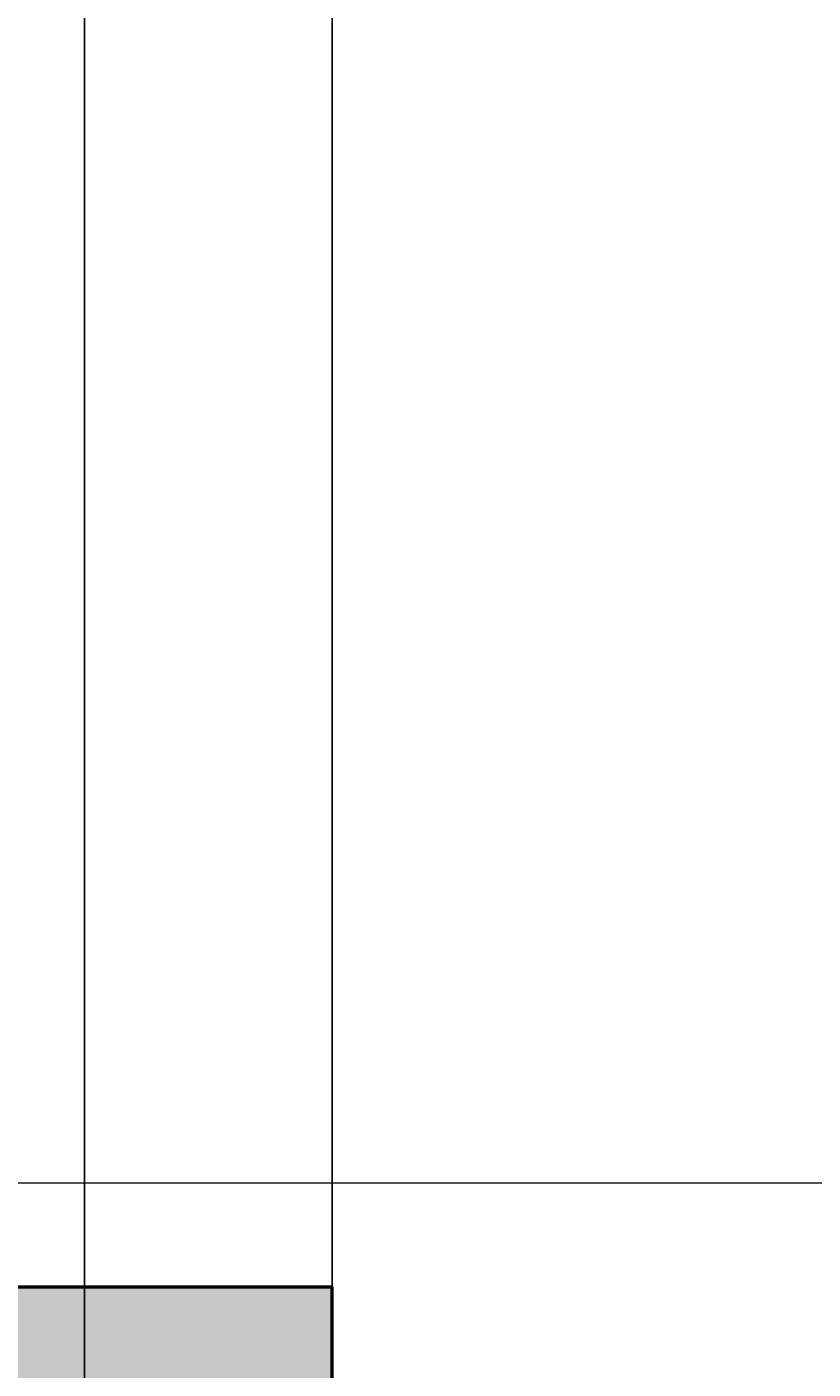
# Model space of a CAD drawing. Units: inches. Extents: x 2231 to 2461, y 2045 to 2455.
# Tile 43 of 95: x 2297 to 2316, y 2185 to 2217. Entities that reach past the tile are written whole.
import ezdxf

# ---------------------------------------------------------------- set-up
doc = ezdxf.new("R2010")
doc.units = ezdxf.units.IN
for name, color, linetype, lineweight in [('A-ANNO-DIMS', 2, 'Continuous', 18), ('A-DOOR', 3, 'Continuous', 25), ('A-FURN', 9, 'Continuous', 18), ('A-WALL', 7, 'Continuous', 50)]:
    doc.layers.add(name, color=color, linetype=linetype, lineweight=lineweight)
doc.layers.add('A-WALL-PATT', color=18, linetype='Continuous', lineweight=13, true_color=0x000000)
doc.styles.get("Standard").update_dxf_attribs({"font": 'arial.ttf'})
doc.dimstyles.get("Standard").update_dxf_attribs({"dimtxt": 0.18, "dimasz": 0.18, "dimexe": 0.18, "dimexo": 0.0625, "dimgap": 0.09, "dimtad": 0, "dimtih": 1, "dimtoh": 1, "dimdec": 4, "dimzin": 0, "dimdsep": 46, "dimtxsty": 'Standard', "dimcen": 0.09, "dimadec": 0, "dimazin": 0, "dimtfac": 1, "dimtdec": 4, "dimtofl": 0, "dimtmove": 0, "dimatfit": 3, "dimfxl": 1, "dimtolj": 1, "dimtzin": 0, "dimarcsym": 0})

# ---------------------------------------------------------------- blocks, each defined once
blk = doc.blocks.new('*U4')
for p, q in [((0, 0), (0, 6)), ((40, 0), (40, 6))]:
    blk.add_line(p, q)
blk.add_lwpolyline([(0, 0), (34.641, -20), (35.516, -18.484), (0.875, 1.516)], close=True)
blk.add_arc((0, 0), 40, 330, 0)
blk = doc.blocks.new('*D49')
at = {"layer": 'A-ANNO-DIMS', "color": 0, "lineweight": -2, "transparency": 16777216}
for p, q in [((2298.794, 2182.895), (2298.794, 2454.645)), ((2304.794, 2182.895), (2304.794, 2454.645)), ((2298.974, 2454.465), (2301.644, 2454.465)), ((2304.614, 2454.465), (2301.943, 2454.465))]:
    blk.add_line(p, q, dxfattribs=at)
at = {"layer": 'A-ANNO-DIMS', "color": 0, "transparency": 16777216}
for points in [[(2298.974, 2454.495), (2298.974, 2454.435), (2298.794, 2454.465)], [(2304.614, 2454.495), (2304.614, 2454.435), (2304.794, 2454.465)]]:
    blk.add_solid(points, dxfattribs=at)
at = {"layer": 'Defpoints', "color": 0, "transparency": 16777216}
for p in [(2304.794, 2454.465), (2298.794, 2182.833), (2304.794, 2182.833)]:
    blk.add_point(p, dxfattribs=at)
at = {"layer": 'A-ANNO-DIMS', "color": 0, "transparency": 16777216, "insert": (2301.794, 2454.465), "char_height": 0.18, "attachment_point": 5}
blk.add_mtext('\\A1;6', dxfattribs=at)
blk = doc.blocks.new('*D50')
at = {"layer": 'A-ANNO-DIMS', "color": 0, "lineweight": -2, "transparency": 16777216}
for p, q in [((2304.794, 2182.895), (2304.794, 2454.645)), ((2334.794, 2182.895), (2334.794, 2454.645)), ((2304.974, 2454.465), (2319.575, 2454.465)), ((2334.614, 2454.465), (2320.012, 2454.465))]:
    blk.add_line(p, q, dxfattribs=at)
at = {"layer": 'A-ANNO-DIMS', "color": 0, "transparency": 16777216}
for points in [[(2304.974, 2454.495), (2304.974, 2454.435), (2304.794, 2454.465)], [(2334.614, 2454.495), (2334.614, 2454.435), (2334.794, 2454.465)]]:
    blk.add_solid(points, dxfattribs=at)
at = {"layer": 'Defpoints', "color": 0, "transparency": 16777216}
for p in [(2334.794, 2454.465), (2304.794, 2182.833), (2334.794, 2182.833)]:
    blk.add_point(p, dxfattribs=at)
at = {"layer": 'A-ANNO-DIMS', "color": 0, "transparency": 16777216, "insert": (2319.794, 2454.465), "char_height": 0.18, "attachment_point": 5}
blk.add_mtext('\\A1;30', dxfattribs=at)
blk = doc.blocks.new('*D51')
at = {"layer": 'A-ANNO-DIMS', "color": 0, "lineweight": -2, "transparency": 16777216}
for p, q in [((2258.794, 2306.77), (2258.794, 2044.803)), ((2330.794, 2306.77), (2330.794, 2044.803)), ((2258.974, 2044.983), (2294.576, 2044.983)), ((2330.614, 2044.983), (2295.011, 2044.983))]:
    blk.add_line(p, q, dxfattribs=at)
at = {"layer": 'A-ANNO-DIMS', "color": 0, "transparency": 16777216}
for points in [[(2258.974, 2045.013), (2258.974, 2044.953), (2258.794, 2044.983)], [(2330.614, 2045.013), (2330.614, 2044.953), (2330.794, 2044.983)]]:
    blk.add_solid(points, dxfattribs=at)
at = {"layer": 'Defpoints', "color": 0, "transparency": 16777216}
for p in [(2258.794, 2306.833), (2330.794, 2306.833), (2330.794, 2044.983)]:
    blk.add_point(p, dxfattribs=at)
at = {"layer": 'A-ANNO-DIMS', "color": 0, "transparency": 16777216, "insert": (2294.794, 2044.983), "char_height": 0.18, "attachment_point": 5}
blk.add_mtext('\\A1;72', dxfattribs=at)
blk = doc.blocks.new('*D65')
at = {"layer": 'A-ANNO-DIMS', "color": 0, "lineweight": -2, "transparency": 16777216}
for p, q in [((2285.635, 2189.285), (2285.635, 2044.803)), ((2340.667, 2189.285), (2340.667, 2044.803)), ((2285.815, 2044.983), (2312.758, 2044.983)), ((2340.487, 2044.983), (2313.545, 2044.983))]:
    blk.add_line(p, q, dxfattribs=at)
at = {"layer": 'A-ANNO-DIMS', "color": 0, "transparency": 16777216}
for points in [[(2285.815, 2045.013), (2285.815, 2044.953), (2285.635, 2044.983)], [(2340.487, 2045.013), (2340.487, 2044.953), (2340.667, 2044.983)]]:
    blk.add_solid(points, dxfattribs=at)
at = {"layer": 'Defpoints', "color": 0, "transparency": 16777216}
for p in [(2285.635, 2189.348), (2340.667, 2189.348), (2340.667, 2044.983)]:
    blk.add_point(p, dxfattribs=at)
at = {"layer": 'A-ANNO-DIMS', "color": 0, "transparency": 16777216, "insert": (2313.151, 2044.983), "char_height": 0.18, "attachment_point": 5}
blk.add_mtext('\\A1;55.03', dxfattribs=at)

msp = doc.modelspace()

# ---------------------------------------------------------------- hatches: boundary and pattern name
at = {"layer": 'A-WALL-PATT'}
h = msp.add_hatch(color=256, dxfattribs=at)
h.dxf.hatch_style = 1
h.paths.add_polyline_path([(2441.7935, 2269.1535), (2432.7935, 2269.1535), (2432.7935, 2186.8328), (2396.7935, 2186.8328), (2396.7935, 2286.8328), (2394.7935, 2286.8328), (2394.7935, 2186.8328), (2334.7935, 2186.8328), (2334.7935, 2182.8328), (2432.7935, 2182.8328), (2432.7935, 2072.8328), (2416.6639, 2072.8328), (2416.6639, 2063.8328), (2441.7935, 2063.8328)])
h.paths.add_polyline_path([(2368.6639, 2072.8328), (2367.04, 2072.8328), (2330.7942, 2072.8328), (2330.7397, 2063.8328), (2368.6639, 2063.8328)])
h.paths.add_polyline_path([(2300.7392, 2068.3328), (2300.7392, 2072.8328), (2298.7935, 2072.8328), (2294.7935, 2072.8328), (2258.7935, 2072.8328), (2258.7935, 2120.8328), (2294.7935, 2120.8328), (2298.7935, 2120.8328), (2298.7935, 2128.8328), (2294.7935, 2128.8328), (2294.7935, 2124.8328), (2258.7935, 2124.8328), (2258.7935, 2182.8328), (2294.7935, 2182.8328), (2294.7935, 2174.8328), (2298.7935, 2174.8328), (2298.7935, 2182.8328), (2304.7935, 2182.8328), (2304.7935, 2186.8328), (2258.7935, 2186.8328), (2258.7935, 2221.999), (2249.7935, 2221.999), (2249.7935, 2063.8328), (2300.7392, 2063.8328)])
h.paths.add_polyline_path([(2391.9338, 2435.8328), (2333.82, 2435.8328), (2333.82, 2426.8328), (2368.7935, 2426.8328), (2368.7935, 2374.9508), (2368.7935, 2370.8328), (2372.3935, 2370.8328), (2372.7935, 2370.8328), (2372.7935, 2426.8328), (2391.9338, 2426.8328)])
h.paths.add_polyline_path([(2441.7935, 2435.8328), (2415.9338, 2435.8328), (2415.9338, 2426.8328), (2432.7935, 2426.8328), (2432.7935, 2334.8328), (2372.7935, 2334.8328), (2372.7935, 2346.8328), (2368.7935, 2346.8328), (2368.7935, 2306.8328), (2360.7935, 2306.8328), (2360.7935, 2302.8328), (2368.7935, 2302.8328), (2372.7935, 2302.8328), (2372.7935, 2330.8328), (2432.7935, 2330.8328), (2432.7935, 2317.1535), (2441.7935, 2317.1535)])
h.paths.add_polyline_path([(2285.82, 2435.8328), (2249.7935, 2435.8328), (2249.7935, 2269.999), (2258.7935, 2269.999), (2258.7935, 2302.8328), (2318.8168, 2302.8328), (2330.7935, 2302.8328), (2330.7935, 2306.8328), (2258.7935, 2306.8328), (2258.7935, 2426.8328), (2285.82, 2426.8328)])

# ---------------------------------------------------------------- linework, layer by layer
at = {"layer": 'A-FURN'}
msp.add_lwpolyline([(2285.6353, 2255.1137), (2285.6353, 2261.3584), (2340.6673, 2261.3584), (2340.6673, 2189.3477), (2285.6353, 2189.3477), (2285.6353, 2195.1137)], dxfattribs=at)
at = {"layer": 'A-WALL'}
for p in [(2258.7935, 2186.8328), (2304.7935, 2182.8328)]:
    msp.add_line(p, (2304.7935, 2186.8328), dxfattribs=at)

# ---------------------------------------------------------------- block references
at = {"layer": 'A-DOOR', "xscale": 0.75, "yscale": 0.75, "zscale": 0.75}
msp.add_blockref('*U4', (2304.7935, 2182.8328), dxfattribs=at)

# ---------------------------------------------------------------- dimensions: what is measured, and where the dimension line sits
at = {"layer": 'A-ANNO-DIMS'}
for base, p1, p2, override, picture, middle in [((2304.7935, 2454.4653), (2298.7935, 2182.8328), (2304.7935, 2182.8328), {"dimdec": 0, "dimlfac": 1, "dimrnd": 0, "dimzin": 0, "dimdsep": 46, "dimlunit": 2}, '*D49', (2301.7935, 2454.4653)), ((2334.7935, 2454.4653), (2304.7935, 2182.8328), (2334.7935, 2182.8328), {"dimdec": 0, "dimlfac": 1, "dimrnd": 0, "dimzin": 0, "dimdsep": 46, "dimlunit": 2}, '*D50', (2319.7935, 2454.4653)), ((2330.7935, 2044.9825), (2258.7935, 2306.8328), (2330.7935, 2306.8328), {"dimdec": 0, "dimlfac": 1, "dimrnd": 0, "dimzin": 0, "dimdsep": 46, "dimlunit": 2}, '*D51', (2294.7935, 2044.9825)), ((2340.6673, 2044.9825), (2285.6353, 2189.3477), (2340.6673, 2189.3477), {"dimdec": 2, "dimlfac": 1, "dimrnd": 0, "dimzin": 0, "dimdsep": 46, "dimlunit": 2}, '*D65', (2313.1513, 2044.9825))]:
    dim = msp.add_linear_dim(base=base, p1=p1, p2=p2, dimstyle='Standard', override=override, dxfattribs=at)
    dim.commit()
    dim.dimension.update_dxf_attribs({"geometry": picture, "text_midpoint": middle})

doc.saveas('drawing.dxf')
